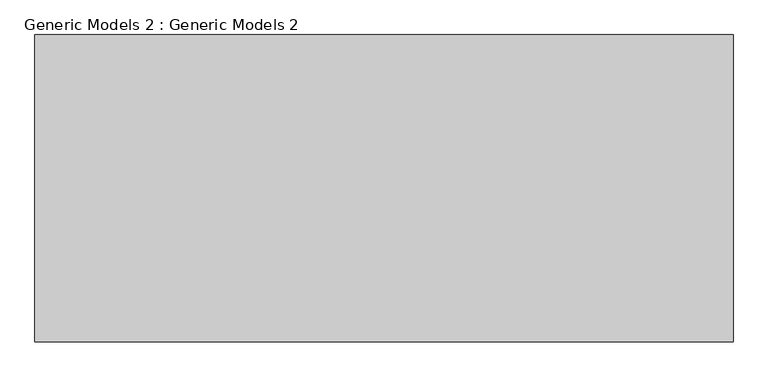
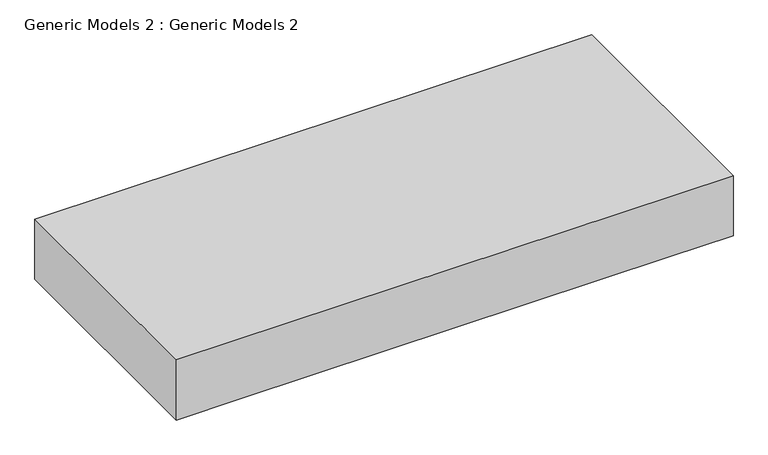
"""IFC4 building model written with IfcOpenShell, lengths in millimetres: proxy geometry, Generic Models 2 : Generic Models 2."""

from ifc_helpers import new_model, si_unit, frame, origin, place, context, project, spatial, polyline, outline, extrude, source, transform, mapped, element, save


def generic_models_2_generic_models_2_5dfb3e49(model_context):
    return source(origin(), model_context, "Body", "SweptSolid", [
        extrude(outline(polyline([(2838.45, -37558.7645004), (2838.45, -37406.3645004), (2838.45, -36377.6645004), (2838.45, -36225.2645004), (2990.85, -36225.2645004), (2990.85, -37558.7645004), (2838.45, -37558.7645004)])), frame((0.0, 5055.615707, 0.0), z_axis=(0.0, 1.0, 0.0), x_axis=(0.0, 0.0, 1.0)), (0.0, 0.0, 1.0), 587.2315015),
    ])


if __name__ == "__main__":
    model = new_model("IFC4")
    model_context = context("Model", 3, world=origin())
    ifc_project = project(units=[si_unit("LENGTHUNIT", "METRE", prefix="MILLI")], contexts=[model_context])
    site = spatial("IfcSite", under=ifc_project)
    building = spatial("IfcBuilding", under=site)
    placement = place(None, origin())
    generic_models_2_generic_models_2_shape = generic_models_2_generic_models_2_5dfb3e49(model_context)
    element("IfcBuildingElementProxy", 1, Name="Generic Models 2 : Generic Models 2", ObjectType="Generic Models 2 : Generic Models 2", at=placement, inside=building, context=model_context, shape_type="MappedRepresentation", body=[
        mapped(generic_models_2_generic_models_2_shape, transform((0.0, 0.0, 0.0), x_axis=(1.0, 0.0, 0.0), y_axis=(0.0, 1.0, 0.0), z_axis=(0.0, 0.0, 1.0))),
    ])
    save(model, "model.ifc")
